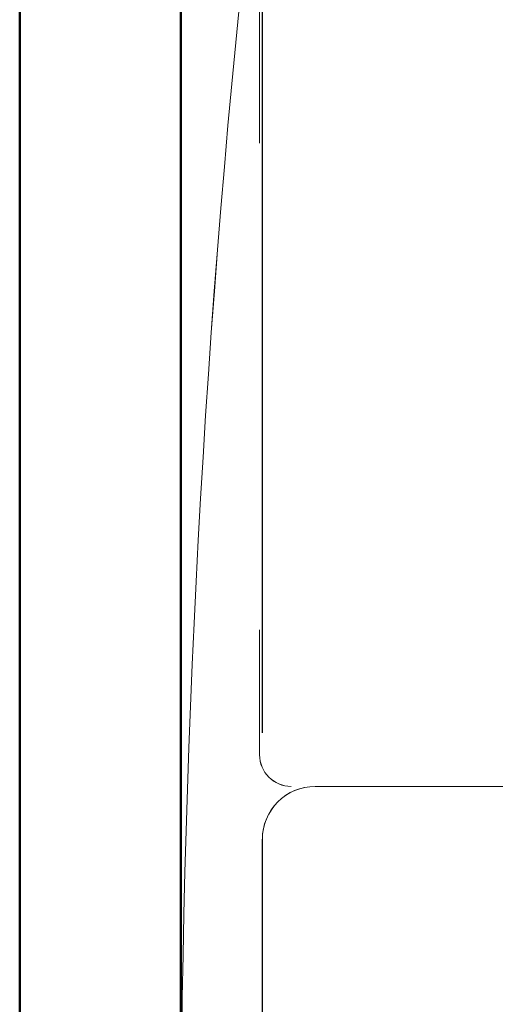
# Model space of a CAD drawing. Units: inches. Extents: x -466983 to 1020, y 324 to 318697.
# Tile 50 of 97: x 609 to 621, y 924 to 949. Entities that reach past the tile are written whole.
import ezdxf

# ---------------------------------------------------------------- set-up
doc = ezdxf.new("R2010")
doc.units = ezdxf.units.IN
doc.header["$MEASUREMENT"] = 0
for name, color, linetype, lineweight in [('A-FLOR-PATT', 252, 'Continuous', 13), ('A-FURN', 8, 'Continuous', 18), ('A-WALL', 7, 'Continuous', 50)]:
    doc.layers.add(name, color=color, linetype=linetype, lineweight=lineweight)

# ---------------------------------------------------------------- blocks, each defined once
blk = doc.blocks.new('L Shaped Sofa')
at = {"ltscale": 2}
for p, q in [((2475.263, 723.229), (2475.263, 821.686)), ((2471.575, 769.955), (2471.575, 802.773)), ((2469.187, 767.567), (2435.071, 767.567)), ((2471.701, 760.482), (2471.701, 766.134)), ((2471.575, 729.305), (2471.575, 765.138)), ((2471.701, 738.472), (2471.701, 736.259)), ((2471.701, 728.35), (2471.701, 736.259))]:
    blk.add_line(p, q, dxfattribs=at)
for centre, radius, start, end in [((1939.075, 785.436), 536.188, 353.68225, 6.54157), ((2469.187, 769.955), 2.388, 270, 0), ((2470.268, 766.134), 1.433, 0, 90)]:
    blk.add_arc(centre, radius, start, end, dxfattribs=at)

msp = doc.modelspace()

# ---------------------------------------------------------------- hatches: boundary and pattern name
at = {"layer": 'A-FLOR-PATT', "transparency": 33554572}
h = msp.add_hatch(dxfattribs=at)
h.set_pattern_fill('ANSI37', color=256, scale=30)
h.set_pattern_definition([(45, (-1212.4137, -290.035), (-2.6516504, 2.6516504), []), (135, (-1212.4137, -290.035), (-2.6516504, -2.6516504), [])])
h.paths.add_polyline_path([(901.806, 1075.938), (900.614, 1075.938), (900.614, 1065.386), (899.391, 1065.386), (898.091, 1065.386), (892.836, 1058.71, -0.258377), (892.188, 1058.351), (879.985, 1058.351, -0.20177), (879.438, 1058.581), (874.081, 1065.386), (872.781, 1065.386), (871.558, 1065.386), (871.558, 1075.938), (813.806, 1075.938), (813.806, 1044.792), (832.395, 1044.792, -0.394795), (848.66, 1028.536), (848.66, 1009.938), (901.806, 1009.938), (901.806, 1015.938), (901.306, 1015.938), (871.306, 1015.938), (871.306, 1017.25), (871.334, 1017.25, -0.401453), (901.306, 1045.938), (901.806, 1045.938)])
edge = h.paths.add_edge_path(flags=16)
edge.add_line((847.773, 1068.949), (847.773, 1073.709))
edge.add_arc((849.227, 1073.709), 1.454, 90, 180, ccw=False)
edge.add_line((849.227, 1075.163), (864.492, 1075.163))
edge.add_arc((864.492, 1073.709), 1.454, 0, 90, ccw=False)
edge.add_line((865.946, 1073.709), (865.946, 1069.004))
edge.add_arc((832.645, 1068.976), 33.301, -20.6123, 0.0472, ccw=False)
edge.add_ellipse((856.859, 1058.48), major_axis=(0, 10.213), ratio=0.685919, start_angle=100.0088, end_angle=259.9912, ccw=False)
edge.add_arc((881.074, 1068.976), 33.301, 180.0472, 200.6123, ccw=False)
h.paths.add_polyline_path([(853.146, 1066.482), (853.146, 1066.453), (853.146, 1066.453, 0.433107), (852.917, 1066.685), (852.917, 1066.453), (853.146, 1066.453), (853.146, 1066.482), (853.088, 1066.612, 0.697939), (852.7, 1066.453), (852.7, 1066.453), (852.7, 1066.482), (852.917, 1067.001), (852.917, 1066.685, -0.396254)], flags=0)
h.paths.add_polyline_path([(861.019, 1066.482), (861.019, 1066.453), (861.019, 1066.453, 0.416404), (860.802, 1066.685), (860.802, 1066.453), (861.019, 1066.453), (861.019, 1066.482), (860.967, 1066.605, 0.713344), (860.573, 1066.453), (860.573, 1066.453), (860.573, 1066.482), (860.802, 1067.001), (860.802, 1066.685, -0.379973)], flags=0)
edge = h.paths.add_edge_path(flags=0)
edge.add_spline(control_points=[(861.13, 1065.785), (861.466, 1065.248), (861.613, 1065.016), (861.983, 1064.374), (862.192, 1063.944), (862.561, 1063.039), (862.721, 1062.563), (862.987, 1061.578), (863.092, 1061.069), (863.245, 1060.031), (863.293, 1059.503), (863.329, 1058.441), (863.318, 1057.908), (863.237, 1056.852), (863.166, 1056.329), (862.97, 1055.308), (862.843, 1054.81), (862.537, 1053.852), (862.357, 1053.393), (861.951, 1052.525), (861.725, 1052.117), (861.233, 1051.362), (860.967, 1051.016), (860.405, 1050.395), (860.108, 1050.12), (859.494, 1049.646), (859.176, 1049.448), (858.528, 1049.13), (858.197, 1049.011), (857.531, 1048.852), (857.196, 1048.812), (856.525, 1048.812), (856.189, 1048.852), (855.524, 1049.01), (855.193, 1049.129), (854.545, 1049.447), (854.227, 1049.645), (853.612, 1050.118), (853.316, 1050.393), (852.753, 1051.014), (852.487, 1051.36), (851.995, 1052.114), (851.769, 1052.523), (851.363, 1053.39), (851.183, 1053.85), (850.877, 1054.807), (850.75, 1055.305), (850.553, 1056.326), (850.483, 1056.849), (850.401, 1057.905), (850.39, 1058.438), (850.426, 1059.5), (850.473, 1060.028), (850.626, 1061.066), (850.732, 1061.575), (850.997, 1062.561), (851.157, 1063.036), (851.525, 1063.942), (851.734, 1064.371), (852.106, 1065.016), (852.254, 1065.25), (852.608, 1065.733)], knot_values=[3.915332, 3.915332, 3.915332, 3.915332, 4.013468, 4.013468, 4.175532, 4.175532, 4.337596, 4.337596, 4.49966, 4.49966, 4.661724, 4.661724, 4.823788, 4.823788, 4.985852, 4.985852, 5.147916, 5.147916, 5.30998, 5.30998, 5.472044, 5.472044, 5.634109, 5.634109, 5.796173, 5.796173, 5.958237, 5.958237, 6.120301, 6.120301, 6.282365, 6.282365, 6.444429, 6.444429, 6.606493, 6.606493, 6.768557, 6.768557, 6.930621, 6.930621, 7.092685, 7.092685, 7.254749, 7.254749, 7.416813, 7.416813, 7.578878, 7.578878, 7.740942, 7.740942, 7.903006, 7.903006, 8.06507, 8.06507, 8.227134, 8.227134, 8.389198, 8.389198, 8.551262, 8.551262, 8.65037, 8.65037, 8.65037, 8.65037], degree=3, periodic=0)
edge.add_line((852.642, 1065.785), (861.13, 1065.785))
edge = h.paths.add_edge_path(flags=0)
edge.add_ellipse((856.85, 1057.743), major_axis=(0, 7.792), ratio=0.687861, start_angle=0, end_angle=360)
h.paths.add_polyline_path([(848.863, 1069.389), (848.863, 1073.96, -0.414214), (849.954, 1075.051), (863.765, 1075.051, -0.414214), (864.856, 1073.96), (864.856, 1069.389, -0.388936), (864.524, 1069.027, -0.043561), (849.195, 1069.027, -0.388936)], flags=0)
h.paths.add_polyline_path([(853.101, 1068.112, -1), (852.677, 1068.112, -1)], flags=0)
edge = h.paths.add_edge_path(flags=0)
edge.add_ellipse((856.859, 1057.338), major_axis=(0, 2.207), ratio=0.657164, start_angle=0, end_angle=360)
h.paths.add_polyline_path([(861.041, 1068.112, -1), (860.618, 1068.112, -1)], flags=0)
edge = h.paths.add_edge_path()
edge.add_line((573.954, 1057.341), (573.954, 1075.938))
edge.add_line((573.954, 1075.938), (558.731, 1075.938))
edge.add_line((558.731, 1075.938), (558.731, 1065.386))
edge.add_line((558.731, 1065.386), (557.507, 1065.386))
edge.add_line((557.507, 1065.386), (556.207, 1065.386))
edge.add_line((556.207, 1065.386), (550.952, 1058.71))
edge.add_arc((550.304, 1059.116), 0.765, 270, 327.9483, ccw=False)
edge.add_line((550.304, 1058.351), (538.101, 1058.351))
edge.add_arc((538.101, 1059.116), 0.765, 224.3704, 270, ccw=False)
edge.add_line((537.555, 1058.581), (532.198, 1065.386))
edge.add_line((532.198, 1065.386), (530.898, 1065.386))
edge.add_line((530.898, 1065.386), (529.674, 1065.386))
edge.add_line((529.674, 1065.386), (529.674, 1075.938))
edge.add_line((529.674, 1075.938), (520.806, 1075.938))
edge.add_line((520.806, 1075.938), (520.806, 1045.938))
edge.add_line((520.806, 1045.938), (521.306, 1045.938))
edge.add_arc((521.306, 1015.938), 30, 2.5075, 90, ccw=False)
edge.add_line((551.277, 1017.25), (551.306, 1017.25))
edge.add_line((551.306, 1017.25), (551.306, 1015.938))
edge.add_line((551.306, 1015.938), (520.806, 1015.938))
edge.add_line((520.806, 1015.938), (520.806, 1009.938))
edge.add_line((520.806, 1009.938), (559.191, 1010.402))
edge.add_arc((559.191, 1011.856), 1.454, 180, 270, ccw=False)
edge.add_line((557.737, 1011.856), (557.737, 1016.561))
edge.add_arc((591.039, 1016.589), 33.301, 159.3877, 180.0472, ccw=False)
edge.add_ellipse((566.824, 1027.085), major_axis=(0, 10.213), ratio=0.685919, start_angle=280.0088, end_angle=439.9912, ccw=False)
edge.add_arc((542.609, 1016.589), 33.301, 0.0472, 20.6123, ccw=False)
edge.add_line((575.91, 1016.616), (575.91, 1011.856))
edge.add_arc((574.456, 1011.856), 1.454, -90, 0, ccw=False)
edge.add_line((574.456, 1010.402), (608.806, 1009.938))
edge.add_line((608.806, 1009.938), (608.806, 1041.086))
edge.add_line((608.806, 1041.086), (590.218, 1041.086))
edge.add_arc((590.775, 1057.907), 16.831, 181.9277, 268.1032, ccw=False)
edge = h.paths.add_edge_path()
edge.add_ellipse((494.244, 583.62), major_axis=(0, 10.213), ratio=0.685919, start_angle=280.0088, end_angle=439.9912, ccw=False)
edge.add_arc((470.03, 573.124), 33.301, 0.0472, 20.6123, ccw=False)
edge.add_line((503.331, 573.152), (503.331, 568.392))
edge.add_arc((501.877, 568.392), 1.454, -90, 0, ccw=False)
edge.add_line((501.877, 566.938), (539.806, 566.938))
edge.add_line((539.806, 566.938), (539.806, 572.938))
edge.add_line((539.806, 572.938), (539.306, 572.938))
edge.add_line((539.306, 572.938), (509.306, 572.938))
edge.add_line((509.306, 572.938), (509.306, 574.25))
edge.add_line((509.306, 574.25), (509.334, 574.25))
edge.add_arc((539.306, 572.938), 30, 90, 177.4925, ccw=False)
edge.add_line((539.306, 602.938), (539.806, 602.938))
edge.add_line((539.806, 602.938), (539.806, 626.938))
edge.add_line((539.806, 626.938), (531.772, 626.938))
edge.add_line((531.772, 626.938), (531.772, 616.386))
edge.add_line((531.772, 616.386), (530.548, 616.386))
edge.add_line((530.548, 616.386), (529.249, 616.386))
edge.add_line((529.249, 616.386), (523.711, 609.351))
edge.add_line((523.711, 609.351), (510.777, 609.351))
edge.add_line((510.777, 609.351), (505.239, 616.386))
edge.add_line((505.239, 616.386), (503.939, 616.386))
edge.add_line((503.939, 616.386), (502.715, 616.386))
edge.add_line((502.715, 616.386), (502.715, 626.938))
edge.add_line((502.715, 626.938), (481.698, 626.938))
edge.add_line((481.698, 626.938), (481.698, 610.995))
edge.add_arc((467.27, 611.473), 14.436, 271.9277, 358.1032, ccw=False)
edge.add_line((467.756, 597.045), (451.806, 597.045))
edge.add_line((451.806, 597.045), (451.806, 584.404))
edge.add_line((451.806, 584.404), (451.806, 566.938))
edge.add_line((451.806, 566.938), (486.612, 566.938))
edge.add_arc((486.612, 568.392), 1.454, 180, 270, ccw=False)
edge.add_line((485.158, 568.392), (485.158, 573.097))
edge.add_arc((518.459, 573.124), 33.301, 159.3877, 180.0472, ccw=False)
h.paths.add_polyline_path([(836.261, 1020.733), (879.89, 1020.733), (879.89, 1039.39), (836.261, 1039.39)], flags=25)
h.paths.add_polyline_path([(549.985, 1036.749), (593.614, 1036.749), (593.614, 1055.407), (549.985, 1055.407)], flags=24)
h.paths.add_polyline_path([(475.123, 595.596), (518.752, 595.596), (518.752, 614.253), (475.123, 614.253)], flags=24)
h = msp.add_hatch(dxfattribs=at)
h.set_pattern_fill('ANSI37', color=256, scale=20)
h.set_pattern_definition([(45, (-1212.4137, -290.035), (-1.767767, 1.767767), []), (135, (-1212.4137, -290.035), (-1.767767, -1.767767), [])])
h.paths.add_polyline_path([(809.806, 870.938), (809.806, 888.152), (806.998, 888.152), (802.662, 888.152), (789.383, 888.152), (786.285, 888.152, -0.414214), (785.499, 888.937), (785.499, 900.196), (785.499, 908.47, -0.414214), (786.808, 909.779, -0.414214), (785.499, 911.088), (785.499, 929.101, -0.414214), (786.808, 930.411, -0.414214), (785.499, 931.72), (785.499, 931.904, -0.414214), (784.19, 930.595), (766.722, 930.595, -0.412359), (765.413, 931.896, -0.413741), (764.115, 930.578), (744.578, 930.422, -0.416556), (743.786, 931.207), (743.786, 933.515), (742.215, 933.515), (742.215, 952.024, -0.001344), (743.786, 952.2), (743.786, 953.938), (678.592, 953.938), (678.592, 951.131), (678.592, 946.794), (678.592, 933.515), (678.592, 930.417, -0.414214), (677.806, 929.631), (666.548, 929.631), (658.274, 929.631, -0.414214), (656.965, 930.94, -0.414214), (655.656, 929.631), (637.642, 929.631, -0.414214), (636.333, 930.94, -0.414214), (635.024, 929.631), (634.839, 929.631, -0.414214), (636.149, 928.322), (636.149, 910.854, -0.412359), (634.848, 909.545, -0.413741), (636.165, 908.247), (636.321, 888.71, -0.416556), (635.536, 887.918), (633.228, 887.918), (633.228, 886.347), (614.719, 886.347, -0.001344), (614.544, 887.918), (612.806, 887.918), (612.806, 834.938), (612.806, 752.938), (612.806, 748.938), (612.806, 697.938), (654.806, 697.938), (654.806, 701.938), (715.806, 701.938), (715.806, 737.435), (774.292, 737.435), (774.292, 795.938), (809.806, 795.938)])
h.paths.add_polyline_path([(679.276, 849.576, 0.102523), (682.148, 849.261, -0.080461), (694.543, 849.773, -0.283899), (694.482, 849.008, 0.136605), (694.407, 848.81, -0.030441), (694.543, 846.893), (694.543, 842.62), (694.543, 838.347, -0.028219), (694.425, 836.568), (694.425, 836.568, 0.196187), (694.446, 836.271, -0.302897), (694.543, 835.467, -0.080461), (682.148, 835.979, 0.102523), (679.276, 835.664, -0.58611), (678.646, 836.017), (678.646, 849.223, -0.58611)], flags=16)
h.paths.add_polyline_path([(679.517, 848.651, 0.699597), (679.476, 848.634, 1.20716), (679.194, 848.742, 0.010621)], flags=0)
h.paths.add_polyline_path([(679.492, 836.561, -0.013798), (679.918, 836.659, -0.071703), (682.853, 837.143, -0.165743), (682.166, 839.101), (682.166, 842.609), (682.166, 846.06, -0.240616), (683.473, 848.677, -0.068263), (693.929, 849.008), (693.788, 848.708), (693.788, 849.023, 0.067332), (683.473, 848.677, 0.240616), (682.166, 846.06), (682.166, 842.609), (682.166, 839.101, 0.23459), (683.461, 836.551, 0.068093), (693.788, 836.195), (693.788, 836.51), (693.93, 836.21, -0.077215), (682.242, 836.782, 0.086627), (679.528, 836.57, -0.628402), (679.503, 836.573), (679.503, 836.607, 0.910458)], flags=0)
h.paths.add_polyline_path([(679.476, 848.636), (679.207, 848.647), (679.207, 836.572, 0.913566), (679.365, 836.586), (679.476, 836.582)], flags=0)
h.paths.add_polyline_path([(679.276, 829.86, 0.102523), (682.148, 829.546, -0.080461), (694.543, 830.057, -0.283899), (694.482, 829.293, 0.136605), (694.407, 829.095, -0.030441), (694.543, 827.178), (694.543, 822.904), (694.543, 818.631, -0.028219), (694.425, 816.853), (694.425, 816.853, 0.196187), (694.446, 816.556, -0.302897), (694.543, 815.752, -0.080461), (682.148, 816.263, 0.102523), (679.276, 815.949, -0.58611), (678.646, 816.302), (678.646, 829.507, -0.58611)], flags=16)
h.paths.add_polyline_path([(679.517, 828.936, 0.699597), (679.476, 828.919, 1.20716), (679.194, 829.027, 0.010621)], flags=0)
h.paths.add_polyline_path([(679.492, 816.846, -0.013798), (679.918, 816.944, -0.071703), (682.853, 817.428, -0.165743), (682.166, 819.385), (682.166, 822.894), (682.166, 826.345, -0.240616), (683.473, 828.961, -0.068263), (693.929, 829.293), (693.788, 828.993), (693.788, 829.308, 0.067332), (683.473, 828.961, 0.240616), (682.166, 826.345), (682.166, 822.894), (682.166, 819.385, 0.23459), (683.461, 816.836, 0.068093), (693.788, 816.48), (693.788, 816.795), (693.93, 816.495, -0.077215), (682.242, 817.066, 0.086627), (679.528, 816.855, -0.628402), (679.503, 816.858), (679.503, 816.892, 0.910458)], flags=0)
h.paths.add_polyline_path([(679.476, 828.921), (679.207, 828.932), (679.207, 816.857, 0.913566), (679.365, 816.871), (679.476, 816.867)], flags=0)
h.paths.add_polyline_path([(679.276, 810.145, 0.102523), (682.148, 809.83, -0.080461), (694.543, 810.342, -0.3023), (694.447, 809.539, 0.10023), (694.406, 809.388, -0.03057), (694.543, 807.462), (694.543, 803.189), (694.543, 798.916, -0.03057), (694.406, 796.991, 0.10023), (694.447, 796.839, -0.3023), (694.543, 796.036, -0.080461), (682.148, 796.548, 0.102523), (679.276, 796.233, -0.58611), (678.646, 796.586), (678.646, 809.792, -0.58611)], flags=16)
h.paths.add_polyline_path([(679.517, 809.242, 0.699597), (679.476, 809.224, 1.20716), (679.194, 809.332, 0.010621)], flags=0)
h.paths.add_polyline_path([(679.492, 797.151, -0.013798), (679.918, 797.25, -0.071703), (682.853, 797.734, -0.165743), (682.166, 799.691), (682.166, 803.2), (682.166, 806.65, -0.239349), (683.461, 809.258, -0.072465), (694.447, 809.541, 0.197932), (694.425, 809.241), (693.788, 809.299), (693.788, 809.614, 0.068093), (683.461, 809.258, 0.239349), (682.166, 806.65), (682.166, 803.2), (682.166, 799.691, 0.235854), (683.473, 797.132, 0.067332), (693.788, 796.786), (693.788, 797.101), (694.425, 797.159, 0.197932), (694.447, 796.859, -0.080419), (682.156, 797.379, 0.083867), (679.528, 797.16, -0.628402), (679.503, 797.164), (679.503, 797.197, 0.910458)], flags=0)
h.paths.add_polyline_path([(679.207, 809.237), (679.207, 797.162, 0.913566), (679.365, 797.176), (679.476, 797.173), (679.476, 809.227)], flags=0)
h.paths.add_polyline_path([(695.364, 853.299), (728.223, 853.299), (728.223, 771.152), (695.364, 771.152)], flags=16)
h.paths.add_polyline_path([(696.021, 852.642), (727.566, 852.642), (727.566, 771.809), (696.021, 771.809)], flags=0)
h.paths.add_polyline_path([(679.276, 788.787, 0.102523), (682.148, 788.472, -0.080461), (694.543, 788.984, -0.3023), (694.447, 788.181, 0.10023), (694.406, 788.03, -0.03057), (694.543, 786.104), (694.543, 781.831), (694.543, 777.558, -0.03057), (694.406, 775.632, 0.10023), (694.447, 775.481, -0.3023), (694.543, 774.678, -0.080461), (682.148, 775.19, 0.102523), (679.276, 774.875, -0.58611), (678.646, 775.228), (678.646, 788.434, -0.58611)], flags=16)
h.paths.add_polyline_path([(679.517, 787.883, 0.699597), (679.476, 787.866, 1.20716), (679.194, 787.974, 0.010621)], flags=0)
h.paths.add_polyline_path([(679.492, 775.793, -0.013798), (679.918, 775.891, -0.071703), (682.853, 776.375, -0.165743), (682.166, 778.333), (682.166, 781.841), (682.166, 785.292, -0.239349), (683.461, 787.899, -0.072465), (694.447, 788.182, 0.197932), (694.425, 787.882), (693.788, 787.94), (693.788, 788.255, 0.068093), (683.461, 787.899, 0.239349), (682.166, 785.292), (682.166, 781.841), (682.166, 778.333, 0.235854), (683.473, 775.774, 0.067332), (693.788, 775.428), (693.788, 775.742), (694.425, 775.8, 0.197932), (694.447, 775.5, -0.080419), (682.156, 776.021, 0.083867), (679.528, 775.802, -0.628402), (679.503, 775.805), (679.503, 775.839, 0.910458)], flags=0)
h.paths.add_polyline_path([(679.207, 787.879), (679.207, 775.804, 0.913566), (679.365, 775.818), (679.476, 775.814), (679.476, 787.868)], flags=0)
h.paths.add_polyline_path([(704.641, 854.12, -0.080461), (705.153, 866.516, 0.102523), (704.838, 869.387, -0.58611), (705.191, 870.017), (718.397, 870.017, -0.58611), (718.75, 869.387, 0.102523), (718.435, 866.516, -0.080461), (718.946, 854.12, -0.3023), (718.144, 854.217, 0.10023), (717.992, 854.257, -0.03057), (716.067, 854.12), (711.794, 854.12), (707.521, 854.12, -0.03057), (705.595, 854.257, 0.10023), (705.444, 854.217, -0.3023)], flags=16)
h.paths.add_polyline_path([(717.846, 869.146, 0.699597), (717.829, 869.187, 1.20716), (717.937, 869.47, 0.010621)], flags=0)
h.paths.add_polyline_path([(705.463, 854.216, -0.080419), (705.984, 866.507, 0.083867), (705.765, 869.135, -0.628402), (705.768, 869.16), (705.802, 869.16, 0.910458), (705.756, 869.171, -0.013798), (705.854, 868.745, -0.071703), (706.338, 865.81, -0.165743), (708.295, 866.497), (711.804, 866.497), (715.255, 866.497, -0.239349), (717.862, 865.202, -0.072465), (718.145, 854.216, 0.197932), (717.845, 854.238), (717.903, 854.876), (718.218, 854.876, 0.068093), (717.862, 865.202, 0.239349), (715.255, 866.497), (711.804, 866.497), (708.295, 866.497, 0.235854), (705.737, 865.19, 0.067332), (705.391, 854.876), (705.705, 854.876), (705.763, 854.238, 0.197932)], flags=16)
h.paths.add_polyline_path([(705.766, 869.456, 0.913566), (705.781, 869.299), (705.777, 869.187), (717.831, 869.187), (717.842, 869.456)], flags=0)
h.paths.add_polyline_path([(729.045, 842.62), (729.045, 846.893, -0.03057), (729.182, 848.818, 0.10023), (729.141, 848.97, -0.3023), (729.045, 849.773, -0.080461), (741.44, 849.261, 0.102523), (744.311, 849.576, -0.58611), (744.942, 849.223), (744.942, 836.017, -0.58611), (744.311, 835.664, 0.102523), (741.44, 835.979, -0.080461), (729.045, 835.467, -0.3023), (729.141, 836.27, 0.10023), (729.182, 836.421, -0.03057), (729.045, 838.347)], flags=16)
h.paths.add_polyline_path([(744.111, 836.585, 1.20716), (744.394, 836.477, 0.010621), (744.07, 836.567, 0.699597)], flags=0)
h.paths.add_polyline_path([(729.141, 836.268, 0.197932), (729.162, 836.568), (729.8, 836.51), (729.8, 836.195, 0.068093), (740.126, 836.551, 0.239349), (741.421, 839.159), (741.421, 842.609), (741.421, 846.118, 0.235854), (740.114, 848.677, 0.067332), (729.8, 849.023), (729.8, 848.708), (729.162, 848.65, 0.197932), (729.141, 848.95, -0.080419), (741.432, 848.43, 0.083867), (744.059, 848.649, -0.628402), (744.085, 848.645), (744.085, 848.612, 0.910458), (744.095, 848.658, -0.013798), (743.67, 848.559, -0.071703), (740.734, 848.075, -0.165743), (741.421, 846.118), (741.421, 842.609), (741.421, 839.159, -0.239349), (740.126, 836.551, -0.072465)], flags=0)
h.paths.add_polyline_path([(729.045, 830.057, -0.080461), (741.44, 829.546, 0.102523), (744.311, 829.86, -0.58611), (744.942, 829.507), (744.942, 816.302, -0.58611), (744.311, 815.949, 0.102523), (741.44, 816.263, -0.080461), (729.045, 815.752, -0.3023), (729.141, 816.554, 0.10023), (729.182, 816.706, -0.03057), (729.045, 818.631), (729.045, 822.904), (729.045, 827.178, -0.03057), (729.182, 829.103, 0.10023), (729.141, 829.255, -0.3023)], flags=16)
h.paths.add_polyline_path([(744.111, 816.869, 1.20716), (744.394, 816.761, 0.010621), (744.07, 816.852, 0.699597)], flags=0)
h.paths.add_polyline_path([(729.141, 829.235, -0.080419), (741.432, 828.714, 0.083867), (744.059, 828.933, -0.628402), (744.085, 828.93), (744.085, 828.896, 0.910458), (744.095, 828.943, -0.013798), (743.67, 828.844, -0.071703), (740.734, 828.36, -0.165743), (741.421, 826.403), (741.421, 822.894), (741.421, 819.443, -0.239349), (740.126, 816.836, -0.072465), (729.141, 816.553, 0.197932), (729.162, 816.853), (729.8, 816.795), (729.8, 816.48, 0.068093), (740.126, 816.836, 0.239349), (741.421, 819.443), (741.421, 822.894), (741.421, 826.403, 0.235854), (740.114, 828.961, 0.067332), (729.8, 829.308), (729.8, 828.993), (729.162, 828.935, 0.197932)], flags=16)
h.paths.add_polyline_path([(729.045, 810.342, -0.080461), (741.44, 809.83, 0.102523), (744.311, 810.145, -0.58611), (744.942, 809.792), (744.942, 796.586, -0.58611), (744.311, 796.233, 0.102523), (741.44, 796.548, -0.080461), (729.045, 796.036, -0.283899), (729.105, 796.801, 0.136605), (729.181, 796.999, -0.030441), (729.045, 798.916), (729.045, 803.189), (729.045, 807.462, -0.028219), (729.163, 809.241), (729.162, 809.241, 0.196187), (729.142, 809.538, -0.302897)], flags=16)
h.paths.add_polyline_path([(744.111, 797.175, 1.20716), (744.394, 797.067, 0.010621), (744.07, 797.158, 0.699597)], flags=0)
h.paths.add_polyline_path([(741.345, 809.027, 0.086627), (744.059, 809.239, -0.628402), (744.085, 809.235), (744.085, 809.202, 0.910458), (744.095, 809.248, -0.013798), (743.67, 809.15, -0.071703), (740.734, 808.666, -0.165743), (741.421, 806.708), (741.421, 803.2), (741.421, 799.749, -0.240616), (740.114, 797.132, -0.068263), (729.658, 796.801), (729.8, 797.101), (729.8, 796.786, 0.067332), (740.114, 797.132, 0.240616), (741.421, 799.749), (741.421, 803.2), (741.421, 806.708, 0.23459), (740.126, 809.258, 0.068093), (729.8, 809.614), (729.8, 809.299), (729.658, 809.599, -0.077215)], flags=0)
h.paths.add_polyline_path([(704.641, 770.33, -0.283899), (705.405, 770.27, 0.136605), (705.603, 770.194, -0.030441), (707.521, 770.33), (711.794, 770.33), (716.067, 770.33, -0.028219), (717.845, 770.212), (717.845, 770.213, 0.196187), (718.143, 770.233, -0.302897), (718.946, 770.33, -0.080461), (718.435, 757.935, 0.102523), (718.75, 755.064, -0.58611), (718.397, 754.433), (705.191, 754.433, -0.58611), (704.838, 755.064, 0.102523), (705.153, 757.935, -0.080461)], flags=16)
h.paths.add_polyline_path([(705.762, 755.305, 0.699597), (705.779, 755.264, 1.20716), (705.671, 754.981, 0.010621)], flags=0)
h.paths.add_polyline_path([(705.405, 769.717), (705.705, 769.575), (705.391, 769.575, 0.067332), (705.737, 759.261, 0.240616), (708.353, 757.954), (711.804, 757.954), (715.313, 757.954, 0.23459), (717.862, 759.249, 0.068093), (718.218, 769.575), (717.903, 769.575), (718.203, 769.717, -0.077215), (717.632, 758.03, 0.086627), (717.843, 755.316, -0.628402), (717.84, 755.29), (717.806, 755.29, 0.910458), (717.853, 755.28, -0.013798), (717.754, 755.705, -0.071703), (717.27, 758.641, -0.165743), (715.313, 757.954), (711.804, 757.954), (708.353, 757.954, -0.240616), (705.737, 759.261, -0.068263)], flags=0)
h.paths.add_polyline_path([(729.045, 788.984, -0.080461), (741.44, 788.472, 0.102523), (744.311, 788.787, -0.58611), (744.942, 788.434), (744.942, 775.228, -0.58611), (744.311, 774.875, 0.102523), (741.44, 775.19, -0.080461), (729.045, 774.678, -0.283899), (729.105, 775.443, 0.136605), (729.181, 775.64, -0.030441), (729.045, 777.558), (729.045, 781.831), (729.045, 786.104, -0.028219), (729.163, 787.882), (729.162, 787.882, 0.196187), (729.142, 788.18, -0.302897)], flags=16)
h.paths.add_polyline_path([(744.111, 775.817, 1.20716), (744.394, 775.709, 0.010621), (744.07, 775.799, 0.699597)], flags=0)
h.paths.add_polyline_path([(741.345, 787.669, 0.086627), (744.059, 787.881, -0.628402), (744.085, 787.877), (744.085, 787.844, 0.910458), (744.095, 787.89, -0.013798), (743.67, 787.791, -0.071703), (740.734, 787.307, -0.165743), (741.421, 785.35), (741.421, 781.841), (741.421, 778.39, -0.240616), (740.114, 775.774, -0.068263), (729.658, 775.443), (729.8, 775.742), (729.8, 775.428, 0.067332), (740.114, 775.774, 0.240616), (741.421, 778.39), (741.421, 781.841), (741.421, 785.35, 0.23459), (740.126, 787.899, 0.068093), (729.8, 788.255), (729.8, 787.94), (729.658, 788.241, -0.077215)], flags=0)
h.paths.add_polyline_path([(744.111, 848.636), (744.111, 836.582), (744.381, 836.572), (744.381, 848.647, 0.913566), (744.223, 848.633)], flags=0)
h.paths.add_polyline_path([(744.223, 828.917), (744.111, 828.921), (744.111, 816.867), (744.381, 816.857), (744.381, 828.932, 0.913566)], flags=0)
h.paths.add_polyline_path([(717.831, 755.264), (705.777, 755.264), (705.766, 754.994), (717.842, 754.994, 0.913566), (717.827, 755.152)], flags=0)
h.paths.add_polyline_path([(744.223, 809.223), (744.111, 809.227), (744.111, 797.173), (744.381, 797.162), (744.381, 809.237, 0.913566)], flags=0)
h.paths.add_polyline_path([(744.111, 787.868), (744.111, 775.814), (744.381, 775.804), (744.381, 787.879, 0.913566), (744.223, 787.865)], flags=0)
h.paths.add_polyline_path([(678.877, 877.123), (737.613, 877.123), (737.613, 899.512), (678.877, 899.512)], flags=24)

# ---------------------------------------------------------------- linework, layer by layer
at = {"layer": 'A-FURN', "ltscale": 2}
for p, q in [((612.806, 953.938), (612.806, 899.962)), ((612.806, 953.938), (612.806, 899.962)), ((612.806, 953.938), (612.806, 899.962)), ((612.806, 953.938), (612.806, 899.962)), ((612.806, 953.938), (612.806, 899.962)), ((612.806, 953.938), (612.806, 899.962)), ((614.758, 951.131), (614.758, 946.794)), ((614.758, 951.131), (614.758, 946.794)), ((614.758, 951.131), (614.758, 946.794)), ((614.758, 951.131), (614.758, 946.794)), ((614.758, 951.131), (614.758, 946.794)), ((614.758, 951.131), (614.758, 946.794)), ((614.827, 950.607), (614.827, 930.963)), ((614.827, 950.607), (614.827, 930.963)), ((614.827, 950.607), (614.827, 930.963)), ((614.827, 950.607), (614.827, 930.963)), ((614.827, 950.607), (614.827, 930.963)), ((614.827, 950.607), (614.827, 930.963)), ((614.758, 945.581), (614.758, 946.794)), ((614.758, 945.581), (614.758, 946.794)), ((614.758, 945.581), (614.758, 946.794)), ((614.758, 945.581), (614.758, 946.794)), ((614.758, 945.581), (614.758, 946.794)), ((614.758, 945.581), (614.758, 946.794)), ((614.758, 933.515), (614.758, 930.417)), ((614.758, 933.515), (614.758, 930.417)), ((614.758, 933.515), (614.758, 930.417)), ((614.758, 933.515), (614.758, 930.417)), ((614.758, 933.515), (614.758, 930.417)), ((614.758, 933.515), (614.758, 930.417)), ((616.137, 929.631), (634.839, 929.631)), ((616.137, 929.631), (634.839, 929.631)), ((616.137, 929.631), (634.839, 929.631)), ((616.137, 929.631), (634.839, 929.631)), ((616.137, 929.631), (634.839, 929.631)), ((616.137, 929.631), (634.839, 929.631)), ((614.827, 928.322), (614.827, 910.331)), ((614.827, 928.322), (614.827, 910.331)), ((614.827, 928.322), (614.827, 910.331)), ((614.827, 928.322), (614.827, 910.331)), ((614.827, 928.322), (614.827, 910.331)), ((614.827, 928.322), (614.827, 910.331))]:
    msp.add_line(p, q, dxfattribs=at)
for centre, radius, start, end in [((906.752, 919.835), 293.946, 173.68225, 186.54157), ((906.752, 919.835), 293.946, 173.68225, 186.54157), ((906.752, 919.835), 293.946, 173.68225, 186.54157), ((906.752, 919.835), 293.946, 173.68225, 186.54157), ((906.752, 919.835), 293.946, 173.68225, 186.54157), ((906.752, 919.835), 293.946, 173.68225, 186.54157), ((615.544, 930.417), 0.785, 180, 270), ((615.544, 930.417), 0.785, 180, 270), ((615.544, 930.417), 0.785, 180, 270), ((615.544, 930.417), 0.785, 180, 270), ((615.544, 930.417), 0.785, 180, 270), ((615.544, 930.417), 0.785, 180, 270), ((616.137, 928.322), 1.309, 90, 180), ((616.137, 928.322), 1.309, 90, 180), ((616.137, 928.322), 1.309, 90, 180), ((616.137, 928.322), 1.309, 90, 180), ((616.137, 928.322), 1.309, 90, 180), ((616.137, 928.322), 1.309, 90, 180)]:
    msp.add_arc(centre, radius, start, end, dxfattribs=at)
at = {"layer": 'A-WALL'}
for p, q in [((608.806, 870.938), (608.806, 1005.938)), ((612.806, 870.938), (612.806, 953.938))]:
    msp.add_line(p, q, dxfattribs=at)

# ---------------------------------------------------------------- block references
at = {"layer": 'A-FURN', "xscale": 0.5482153745360612, "yscale": 0.5482153745360612, "zscale": 0.5482153745360612, "rotation": 180}
msp.add_blockref('L Shaped Sofa', (1969.783, 1350.423), dxfattribs=at)

doc.saveas('drawing.dxf')
